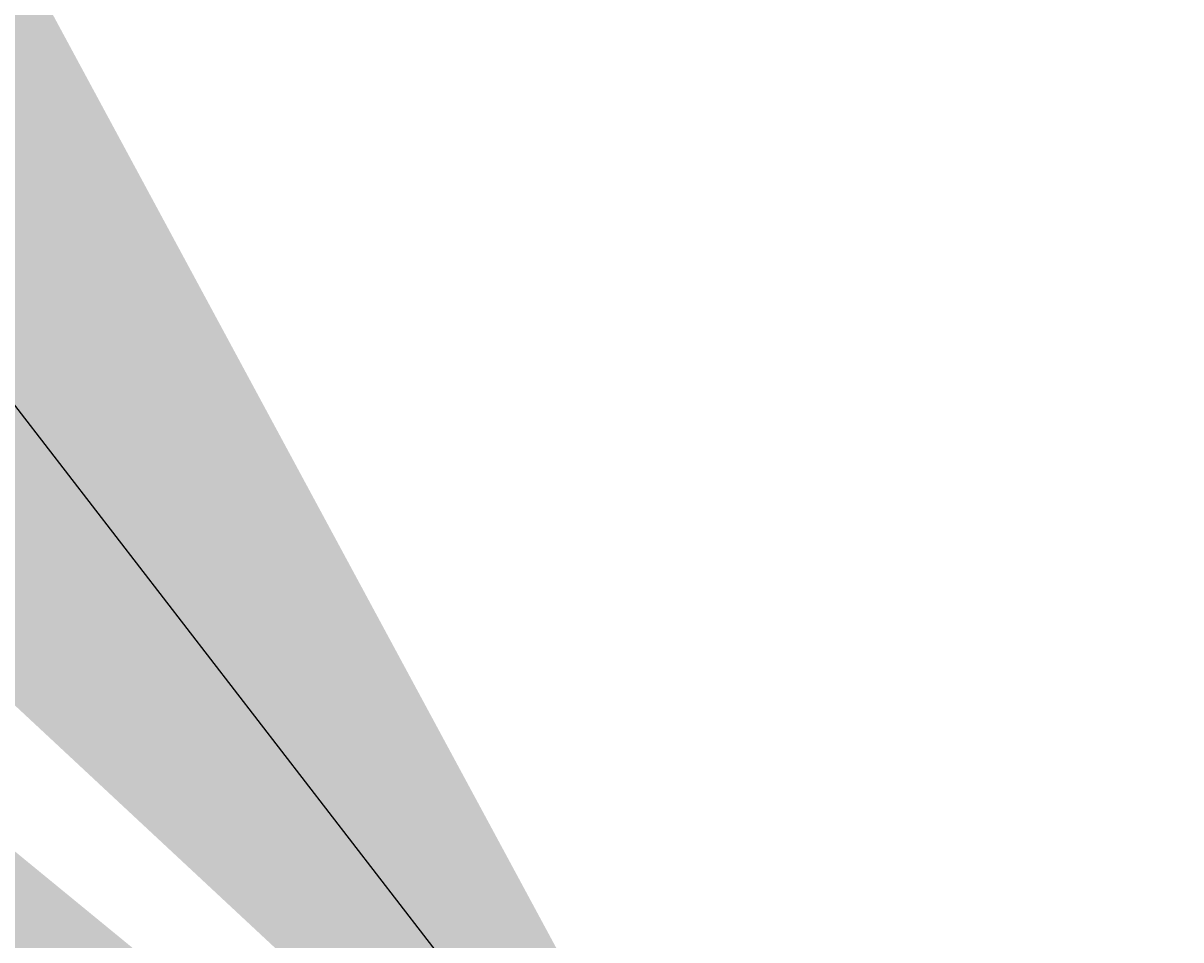
# Model space of a CAD drawing. Units: inches. Extents: x -9413 to 9703, y -9719 to 9096.
# Tile 1 of 1: x -993 to 493, y 865 to 2041. Entities that reach past the tile are written whole.
import ezdxf
from ezdxf import colors
from ezdxf.entities.mleader import LeaderData, LeaderLine
from ezdxf.math import Vec2, Vec3

# ---------------------------------------------------------------- set-up
doc = ezdxf.new("R2010")
doc.units = ezdxf.units.IN
doc.header["$MEASUREMENT"] = 0
doc.layers.add('M-ANNO-TEXT', color=7, linetype='Continuous', lineweight=18)
doc.styles.get("Standard").update_dxf_attribs({"font": 'arial.ttf'})

msp = doc.modelspace()

# ---------------------------------------------------------------- leaders
at = {"layer": 'M-ANNO-TEXT'}
ml = msp.add_multileader_mtext('Standard', dxfattribs=at)
ml.set_content('steam drum', color=256)
ml.set_leader_properties()
ml.build(insert=Vec2(0, 0))
ml.multileader.update_dxf_attribs({"dogleg_length": 0.36, "arrow_head_size": 10000, "scale": 10})
ctx = ml.context
ctx.base_point, ctx.scale, ctx.char_height, ctx.arrow_head_size, ctx.landing_gap_size, ctx.plane_origin = Vec3(1.078100315116472, 187.1657656808087), 10, 5.4, 10000, 0.9, Vec3(56.53630785249729, 178.1917761520126)
ctx.text_align_type = 2
notes = []
notes.append((ctx, [(0, (1, 1, 0), (49.60206616053652, 187.1657656808087), (-1, 0), 7.616326009130828, [(0, [(56.5363078524973, 178.1917761520126)], 0, [])])]))
ctx.mtext.insert, ctx.mtext.alignment, ctx.mtext.flow_direction = Vec3(41.08574015140569, 189.9099675907678), 3, 5
ml = msp.add_multileader_mtext('Standard', dxfattribs=at)
ml.set_content('Reheater', color=256)
ml.set_leader_properties()
ml.build(insert=Vec2(0, 0))
ml.multileader.update_dxf_attribs({"dogleg_length": 0.36, "arrow_head_size": 10000, "scale": 10})
ctx = ml.context
ctx.base_point, ctx.scale, ctx.char_height, ctx.arrow_head_size, ctx.landing_gap_size, ctx.plane_origin = Vec3(234.1414050860131, 159.7303554673012), 10, 5.4, 10000, 0.9, Vec3(221.1444910066821, 154.3050445940477)
notes.append((ctx, [(0, (1, 1, 0), (230.5414050860131, 159.7303554673012), (1, 0), 3.599999999999999, [(0, [(221.1444910066821, 154.3050445940477)], 0, [])])]))
ctx.mtext.insert, ctx.mtext.flow_direction = Vec3(235.0414050860131, 162.4745573772603), 5
ml = msp.add_multileader_mtext('Standard', dxfattribs=at)
ml.set_content('Boiler', color=256)
ml.set_leader_properties()
ml.build(insert=Vec2(0, 0))
ml.multileader.update_dxf_attribs({"dogleg_length": 0.36, "arrow_head_size": 10000, "scale": 10})
ctx = ml.context
ctx.base_point, ctx.scale, ctx.char_height, ctx.arrow_head_size, ctx.landing_gap_size, ctx.plane_origin = Vec3(31.04430257849453, 103.0991380116177), 10, 5.4, 10000, 0.9, Vec3(69.11352005531556, 99.3051261342938)
ctx.text_align_type = 2
notes.append((ctx, [(0, (1, 1, 0), (62.54209871927075, 103.0991380116177), (-1, 0), 10.86041551321825, [(0, [(69.11352005531556, 99.3051261342938)], 0, [])])]))
ctx.mtext.insert, ctx.mtext.alignment, ctx.mtext.flow_direction = Vec3(50.7816832060525, 105.8433399215768), 3, 5
for ctx, leaders in notes:
    for number, flags, end, landing, length, lines in leaders:
        leader = LeaderData()
        leader.index, (leader.has_last_leader_line, leader.has_dogleg_vector, leader.attachment_direction) = number, flags
        leader.last_leader_point, leader.dogleg_vector, leader.dogleg_length = Vec3(end), Vec3(landing), length
        for number, points, colour, breaks in lines:
            line = LeaderLine()
            line.index, line.vertices, line.color, line.breaks = number, Vec3.list(points), colors.encode_raw_color(colour), breaks
            leader.lines.append(line)
        ctx.leaders.append(leader)

doc.saveas('drawing.dxf')
